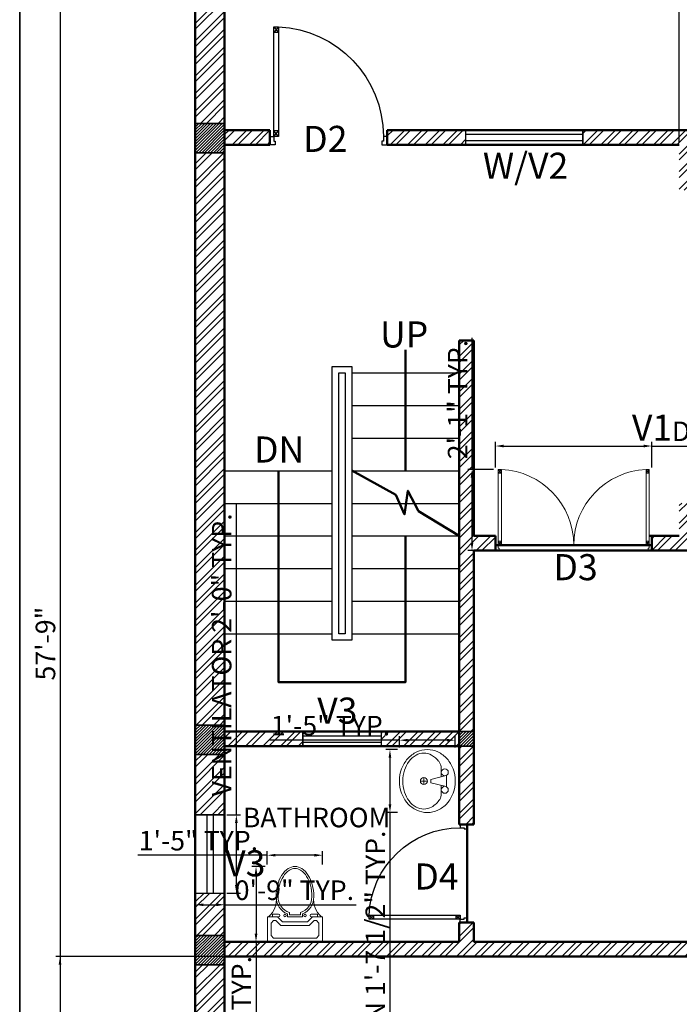
# Model space of a CAD drawing. Units: millimetres. Extents: x 20768 to 23556, y 50760 to 52704.
# Tile 24 of 36: x 21272 to 21474, y 52066 to 52368. Entities that reach past the tile are written whole.
import ezdxf

# ---------------------------------------------------------------- set-up
doc = ezdxf.new("R2010")
doc.units = ezdxf.units.MM
for name, color, linetype, lineweight in [('A-ANNO-TTLB', 7, 'Continuous', 35), ('A-AREA-IDEN', 40, 'Continuous', 18), ('A-DOOR', 3, 'Continuous', 25), ('A-FLOR-STRS', 11, 'Continuous', 25), ('A-FURN', 8, 'Continuous', 18), ('A-GLAZ', 4, 'Continuous', 25), ('A-WALL', 7, 'Continuous', 50), ('A-WALL-PATT', 8, 'Continuous', 13), ('S-ANNO-DIMS', 2, 'Continuous', 18), ('S-COLS', 20, 'Continuous', 35)]:
    doc.layers.add(name, color=color, linetype=linetype, lineweight=lineweight)
doc.styles.get("Standard").update_dxf_attribs({"font": 'arial.ttf'})
doc.dimstyles.new('ISO-25', dxfattribs={"dimtxt": 6, "dimasz": 2.5, "dimexe": 1.25, "dimexo": 0.625, "dimtad": 1, "dimdec": 0, "dimlunit": 3, "dimtxsty": 'Standard', "dimcen": 2.5, "dimadec": 0, "dimazin": 0, "dimtfac": 1, "dimtdec": 0, "dimtmove": 0, "dimatfit": 3, "dimfxl": 1, "dimarcsym": 0})
pattern_1 = [(45, (345.4904, 0), (-0.449012806, 0.449012806), [])]
pattern_2 = [(45, (-37.4434, 0), (-2.69407684, 2.69407684), []), (45, (-35.6473, 0), (-2.69407684, 2.69407684), [])]

# ---------------------------------------------------------------- blocks, each defined once
blk = doc.blocks.new('Puerta 01')
for p, q in [((-0.7745, -0.0264), (-0.7368, -0.0584)), ((-0.7745, -0.0584), (-0.7368, -0.0264)), ((-0.7368, -0.0584), (-0.7368, -0.0264)), ((-0.028, -0.0584), (-0.0657, -0.0264)), ((-0.028, -0.0264), (-0.0657, -0.0584)), ((-0.0657, -0.0584), (-0.0657, -0.0264))]:
    blk.add_line(p, q)
for points in [[(-0.028, 0), (-0.028, -0.0264), (0.004, -0.0264), (0.004, -0.036), (0.028, -0.036), (0.028, 0)], [(-0.028, -0.0264), (-0.7745, -0.0264), (-0.7745, -0.0584), (-0.028, -0.0584)], [(0.004, -0.7736), (0.004, -0.764), (0.028, -0.764), (0.028, -0.8), (-0.028, -0.8), (-0.028, -0.7736)]]:
    blk.add_lwpolyline(points, close=True)
blk.add_arc((-0.028, -0.0264), 0.7472, 182.45453, 270)
blk = doc.blocks.new('md')
for p, q in [((21281.56, 52416.74), (21282.55, 52415.57)), ((21282.55, 52416.74), (21281.56, 52415.57)), ((21327.92, 52416.74), (21326.93, 52415.57)), ((21326.93, 52416.74), (21327.92, 52415.57)), ((21282.55, 52415.57), (21281.56, 52415.57)), ((21326.93, 52415.57), (21327.92, 52415.57)), ((21282.55, 52393.58), (21281.56, 52394.75)), ((21281.56, 52393.58), (21282.55, 52394.75)), ((21282.55, 52394.75), (21281.56, 52394.75)), ((21326.93, 52393.58), (21327.92, 52394.75)), ((21327.92, 52393.58), (21326.93, 52394.75)), ((21326.93, 52394.75), (21327.92, 52394.75))]:
    blk.add_line(p, q)
for points in [[(21281.56, 52393.58), (21281.56, 52416.74), (21282.55, 52416.74), (21282.55, 52393.58)], [(21327.92, 52393.58), (21327.92, 52416.74), (21326.93, 52416.74), (21326.93, 52393.58)], [(21280.74, 52393.58), (21281.56, 52393.58), (21281.56, 52392.59), (21281.86, 52392.59), (21281.86, 52391.84), (21280.74, 52391.84)], [(21328.74, 52393.58), (21327.92, 52393.58), (21327.92, 52392.59), (21327.62, 52392.59), (21327.62, 52391.84), (21328.74, 52391.84)]]:
    blk.add_lwpolyline(points, close=True)
for centre, start, end in [((21281.56, 52393.58), 0, 87.5455), ((21327.92, 52393.58), 92.4545, 180)]:
    blk.add_arc(centre, 23.18, start, end)
blk = doc.blocks.new('A$C0E746A5D')
for p, q in [((0.1052, 0.332), (0.1052, 0.2695)), ((0.0657, 0.276), (0.0657, 0.1972)), ((0.0789, 0.276), (0.184, 0.2497)), ((0.184, 0.2235), (0.0789, 0.1972)), ((0.184, 0.2497), (0.184, 0.2235)), ((0.2103, 0.2366), (0.2629, 0.2366)), ((0.2366, 0.2629), (0.2366, 0.2103)), ((0.1052, 0.2037), (0.1052, 0.141))]:
    blk.add_line(p, q)
for centre in [(0.0789, 0.3023), (0.2366, 0.2366), (0.0789, 0.1709)]:
    blk.add_circle(centre, 0.0263)
for centre, radius, start, end in [((0.2214, 0.2619), 0.2138, 114.98506, 138.36645), ((0.2103, 0.2856), 0.1876, 89.99999, 114.98508), ((0.2366, 0.3272), 0.1197, 90, 118.9112), ((0.2103, 0.2856), 0.1876, 65.01492, 90.00001), ((0.2366, 0.3272), 0.1197, 61.0888, 90), ((0.1992, 0.2619), 0.2138, 41.63355, 65.01494), ((0.2386, 0.2465), 0.2368, 138.36645, 159.7868), ((0.184, 0.332), 0.0789, 147.74019, 180), ((0.2607, 0.2836), 0.1695, 118.9112, 147.74019), ((0.2125, 0.2836), 0.1695, 36.8699, 61.0888), ((0.1746, 0.2552), 0.2169, 17.25794, 36.8699), ((0.182, 0.2465), 0.2368, 20.2132, 41.63355), ((0.2656, 0.2366), 0.2656, 159.78682, 180), ((0.1148, 0.2366), 0.2795, 0, 17.25794), ((0.155, 0.2366), 0.2656, 0, 20.21318), ((0.2656, 0.2366), 0.2656, 180, 200.21318), ((0.1148, 0.2366), 0.2795, 342.74206, 0), ((0.155, 0.2366), 0.2656, 339.78682, 360), ((0.1746, 0.218), 0.2169, 323.1301, 342.74206), ((0.2386, 0.2267), 0.2368, 200.2132, 221.63355), ((0.184, 0.141), 0.0789, 180, 213.90451), ((0.2986, 0.218), 0.2169, 213.90451, 216.8699), ((0.2607, 0.1896), 0.1695, 216.8699, 241.0888), ((0.2125, 0.1896), 0.1695, 298.9112, 323.1301), ((0.182, 0.2267), 0.2368, 318.36645, 339.7868), ((0.2214, 0.2113), 0.2138, 221.63355, 245.01494), ((0.2103, 0.1876), 0.1876, 245.01492, 270.00001), ((0.2366, 0.146), 0.1197, 241.0888, 270), ((0.2103, 0.1876), 0.1876, 269.99999, 294.98508), ((0.2366, 0.146), 0.1197, 270, 298.9112), ((0.1992, 0.2113), 0.2138, 294.98506, 318.36645)]:
    blk.add_arc(centre, radius, start, end)
blk = doc.blocks.new('A$C098B081F')
for p, q in [((558.8, 762), (0, 762)), ((0, 762), (0, 508)), ((63.5, 723.9), (38.1, 698.5)), ((38.1, 698.5), (38.1, 571.5)), ((495.3, 723.9), (63.5, 723.9)), ((520.7, 698.5), (495.3, 723.9)), ((520.7, 698.5), (520.7, 571.5)), ((558.8, 762), (558.8, 508)), ((136.6, 596.9), (85.8, 546.1)), ((422.2, 596.9), (136.6, 596.9)), ((422.2, 596.9), (473, 546.1)), ((0, 508), (12.7, 508)), ((12.7, 508), (101.6, 508)), ((38.1, 571.5), (63.5, 546.1)), ((50.8, 508), (50.8, 482.6)), ((50.8, 508), (101.6, 508)), ((63.5, 546.1), (85.8, 546.1)), ((152.4, 558.8), (101.6, 508)), ((114.3, 508), (101.6, 508)), ((406.4, 558.8), (152.4, 558.8)), ((203.2, 508), (203.2, 479.4)), ((203.2, 508), (355.6, 508)), ((355.6, 508), (355.6, 479.4)), ((406.4, 558.8), (457.2, 508)), ((444.5, 508), (457.2, 508)), ((508, 508), (457.2, 508)), ((495.3, 546.1), (473, 546.1)), ((495.3, 546.1), (520.7, 571.5)), ((508, 508), (546.1, 508)), ((508, 508), (508, 482.6)), ((558.8, 508), (546.1, 508)), ((50.8, 482.6), (114.3, 482.6)), ((223.2, 488), (223.2, 465.8)), ((223.2, 488), (335.6, 488)), ((335.6, 488), (335.6, 465.8)), ((508, 482.6), (444.5, 482.6))]:
    blk.add_line(p, q)
for centre in [(177.8, 495.3), (381, 495.3)]:
    blk.add_circle(centre, 12.7)
for centre, radius, start, end in [((-137.5, 335.8), 228.5, 352.20108, 48.91101), ((114.3, 495.3), 12.7, 270, 90), ((444.5, 495.3), 12.7, 90, 270), ((696.3, 335.8), 228.5, 131.08899, 187.79892), ((279.4, 304.8), 190.5, 113.57818, 180), ((279.4, 304.8), 170.5, 109.24564, 180), ((279.4, 304.8), 170.5, 0, 70.75436), ((279.4, 304.8), 190.5, 0, 66.42182), ((574.9, 304.8), 486, 180.00004, 194.51425), ((574.9, 304.8), 466, 180.00004, 194.51425), ((-16.1, 304.8), 466, 345.48575, 359.99996), ((-16.1, 304.8), 486, 345.48575, 359.99996), ((429.2, 267.1), 335.5, 194.51426, 212.00539), ((429.2, 267.1), 315.5, 194.51426, 212.00539), ((337.2, 209.6), 207, 212.00541, 236.46588), ((221.6, 209.6), 207, 303.53412, 327.99459), ((129.6, 267.1), 315.5, 327.99461, 345.48574), ((129.6, 267.1), 335.5, 327.99461, 345.48574), ((337.2, 209.6), 227, 212.00541, 236.46588), ((279.4, 122.4), 122.4, 236.46593, 269.99995), ((279.4, 122.4), 102.4, 236.46593, 269.99995), ((279.4, 122.4), 102.4, 270.00005, 303.53407), ((279.4, 122.4), 122.4, 270.00005, 303.53407), ((221.6, 209.6), 227, 303.53412, 327.99459)]:
    blk.add_arc(centre, radius, start, end)
blk = doc.blocks.new('WIN-PLAN-A')
blk.add_line((36, 4.5), (36, 0))
blk.add_lwpolyline([(36, 4.5), (0, 4.5), (0, 0), (36, 0)], close=True)
blk = doc.blocks.new('WIN-PLAN-B')
blk.add_line((0, 4.5), (0, 0))
blk.add_lwpolyline([(0, 4.5), (24, 4.5), (24, 0), (0, 0)], close=True)
blk = doc.blocks.new('WIN-PLAN-D')
blk.add_line((0, 24), (9, 24))
blk.add_lwpolyline([(9, 24), (0, 24), (0, 0), (9, 0)], close=True)
blk = doc.blocks.new('*D181')
at = {"layer": 'Defpoints', "color": 0, "transparency": 16777216}
for p in [(21334.74, 52123.9), (21338.34, 52123.9), (21334.74, 52099.9)]:
    blk.add_point(p, dxfattribs=at)
at = {"layer": 'S-ANNO-DIMS', "color": 0, "lineweight": -2, "transparency": 16777216}
for p, q in [((21338.34, 52123.9), (21338.34, 52219.49)), ((21335.37, 52123.9), (21339.59, 52123.9)), ((21338.34, 52102.4), (21338.34, 52121.4)), ((21335.37, 52099.9), (21339.59, 52099.9))]:
    blk.add_line(p, q, dxfattribs=at)
at = {"layer": 'S-ANNO-DIMS', "color": 0, "transparency": 16777216}
for points in [[(21337.92, 52121.4), (21338.76, 52121.4), (21338.34, 52123.9)], [(21337.92, 52102.4), (21338.76, 52102.4), (21338.34, 52099.9)]]:
    blk.add_solid(points, dxfattribs=at)
at = {"layer": 'S-ANNO-DIMS', "color": 0, "transparency": 16777216, "insert": (21334.61, 52172.94), "char_height": 6, "attachment_point": 5, "rotation": 90}
blk.add_mtext('VENTILATOR 2\'-0" TYP.', dxfattribs=at)
blk = doc.blocks.new('*D182')
at = {"layer": 'Defpoints', "color": 0, "transparency": 16777216}
for p in [(21325.74, 52099.9), (21334.74, 52099.9), (21334.74, 52096.3)]:
    blk.add_point(p, dxfattribs=at)
at = {"layer": 'S-ANNO-DIMS', "color": 0, "lineweight": -2, "transparency": 16777216}
for p, q in [((21325.74, 52099.27), (21325.74, 52095.05)), ((21334.74, 52099.27), (21334.74, 52095.05)), ((21328.24, 52096.3), (21332.24, 52096.3)), ((21334.74, 52096.3), (21375.06, 52096.3))]:
    blk.add_line(p, q, dxfattribs=at)
at = {"layer": 'S-ANNO-DIMS', "color": 0, "transparency": 16777216}
for points in [[(21328.24, 52096.71), (21328.24, 52095.88), (21325.74, 52096.3)], [(21332.24, 52096.71), (21332.24, 52095.88), (21334.74, 52096.3)]]:
    blk.add_solid(points, dxfattribs=at)
at = {"layer": 'S-ANNO-DIMS', "color": 0, "transparency": 16777216, "insert": (21356.15, 52099.99), "char_height": 6, "attachment_point": 5}
blk.add_mtext('0\'-9" TYP.', dxfattribs=at)
blk = doc.blocks.new('*D185')
at = {"layer": 'Defpoints', "color": 0, "transparency": 16777216}
for p in [(21465.84, 52236.99), (21417.84, 52229.79), (21465.84, 52229.79)]:
    blk.add_point(p, dxfattribs=at)
at = {"layer": 'S-ANNO-DIMS', "color": 0, "lineweight": -2, "transparency": 16777216}
for p, q in [((21417.84, 52230.42), (21417.84, 52238.24)), ((21465.84, 52230.42), (21465.84, 52238.24)), ((21420.34, 52236.99), (21463.34, 52236.99)), ((21465.84, 52236.99), (21583.18, 52236.99))]:
    blk.add_line(p, q, dxfattribs=at)
at = {"layer": 'S-ANNO-DIMS', "color": 0, "transparency": 16777216}
for points in [[(21420.34, 52237.41), (21420.34, 52236.58), (21417.84, 52236.99)], [(21463.34, 52237.41), (21463.34, 52236.58), (21465.84, 52236.99)]]:
    blk.add_solid(points, dxfattribs=at)
at = {"layer": 'S-ANNO-DIMS', "color": 0, "transparency": 16777216, "insert": (21525.76, 52240.73), "char_height": 6, "attachment_point": 5}
blk.add_mtext('DOUBLE DOOR D3 4\'-0" TYP.', dxfattribs=at)
blk = doc.blocks.new('*D186')
at = {"layer": 'Defpoints', "color": 0, "transparency": 16777216}
for p in [(21410.64, 52229.79), (21417.84, 52229.79), (21417.84, 52204.9)]:
    blk.add_point(p, dxfattribs=at)
at = {"layer": 'S-ANNO-DIMS', "color": 0, "lineweight": -2, "transparency": 16777216}
for p, q in [((21410.64, 52229.79), (21410.64, 52270.22)), ((21417.21, 52229.79), (21409.39, 52229.79)), ((21410.64, 52207.4), (21410.64, 52227.29)), ((21417.21, 52204.9), (21409.39, 52204.9))]:
    blk.add_line(p, q, dxfattribs=at)
at = {"layer": 'S-ANNO-DIMS', "color": 0, "transparency": 16777216}
for points in [[(21410.22, 52227.29), (21411.05, 52227.29), (21410.64, 52229.79)], [(21410.22, 52207.4), (21411.05, 52207.4), (21410.64, 52204.9)]]:
    blk.add_solid(points, dxfattribs=at)
at = {"layer": 'S-ANNO-DIMS', "color": 0, "transparency": 16777216, "insert": (21407, 52251.26), "char_height": 6, "attachment_point": 5, "rotation": 90}
blk.add_mtext('2\'-1" TYP.', dxfattribs=at)
blk = doc.blocks.new('*D197')
at = {"layer": 'Defpoints', "color": 0, "transparency": 16777216}
for p in [(21388.36, 52143.88), (21385.47, 52124.58), (21388.36, 52124.58)]:
    blk.add_point(p, dxfattribs=at)
at = {"layer": 'S-ANNO-DIMS', "color": 0, "lineweight": -2, "transparency": 16777216}
for p, q in [((21387.74, 52143.88), (21384.22, 52143.88)), ((21385.47, 52141.38), (21385.47, 52127.08)), ((21387.74, 52124.58), (21384.22, 52124.58)), ((21385.47, 52124.58), (21385.47, 52015.08))]:
    blk.add_line(p, q, dxfattribs=at)
at = {"layer": 'S-ANNO-DIMS', "color": 0, "transparency": 16777216}
for points in [[(21385.05, 52141.38), (21385.88, 52141.38), (21385.47, 52143.88)], [(21385.05, 52127.08), (21385.88, 52127.08), (21385.47, 52124.58)]]:
    blk.add_solid(points, dxfattribs=at)
at = {"layer": 'S-ANNO-DIMS', "color": 0, "transparency": 16777216, "insert": (21381.74, 52068.58), "char_height": 6, "attachment_point": 5, "rotation": 90}
blk.add_mtext('WASH BASIN 1\'-7 1/2" TYP.', dxfattribs=at)
blk = doc.blocks.new('*D198')
at = {"layer": 'Defpoints', "color": 0, "transparency": 16777216}
for p in [(21388.36, 52146.77), (21388.36, 52143.88), (21405.51, 52143.88)]:
    blk.add_point(p, dxfattribs=at)
at = {"layer": 'S-ANNO-DIMS', "color": 0, "lineweight": -2, "transparency": 16777216}
for p, q in [((21388.36, 52144.5), (21388.36, 52148.02)), ((21405.51, 52144.5), (21405.51, 52148.02)), ((21388.36, 52146.77), (21348.6, 52146.77)), ((21403.01, 52146.77), (21390.86, 52146.77))]:
    blk.add_line(p, q, dxfattribs=at)
at = {"layer": 'S-ANNO-DIMS', "color": 0, "transparency": 16777216}
for points in [[(21390.86, 52147.19), (21390.86, 52146.36), (21388.36, 52146.77)], [(21403.01, 52147.19), (21403.01, 52146.36), (21405.51, 52146.77)]]:
    blk.add_solid(points, dxfattribs=at)
at = {"layer": 'S-ANNO-DIMS', "color": 0, "transparency": 16777216, "insert": (21367.23, 52150.46), "char_height": 6, "attachment_point": 5}
blk.add_mtext('1\'-5" TYP.', dxfattribs=at)
blk = doc.blocks.new('*D199')
at = {"layer": 'Defpoints', "color": 0, "transparency": 16777216}
for p in [(21347.84, 52108.03), (21344.37, 52084.9), (21347.84, 52084.9)]:
    blk.add_point(p, dxfattribs=at)
at = {"layer": 'S-ANNO-DIMS', "color": 0, "lineweight": -2, "transparency": 16777216}
for p, q in [((21347.22, 52108.03), (21343.12, 52108.03)), ((21344.37, 52105.53), (21344.37, 52087.4)), ((21347.22, 52084.9), (21343.12, 52084.9)), ((21344.37, 52084.9), (21344.37, 52023.37))]:
    blk.add_line(p, q, dxfattribs=at)
at = {"layer": 'S-ANNO-DIMS', "color": 0, "transparency": 16777216}
for points in [[(21343.96, 52105.53), (21344.79, 52105.53), (21344.37, 52108.03)], [(21343.96, 52087.4), (21344.79, 52087.4), (21344.37, 52084.9)]]:
    blk.add_solid(points, dxfattribs=at)
at = {"layer": 'S-ANNO-DIMS', "color": 0, "transparency": 16777216, "insert": (21340.65, 52052.89), "char_height": 6, "attachment_point": 5, "rotation": 90}
blk.add_mtext('WC 1\'-11" TYP.', dxfattribs=at)
blk = doc.blocks.new('*D200')
at = {"layer": 'Defpoints', "color": 0, "transparency": 16777216}
for p in [(21347.84, 52111.5), (21347.84, 52108.03), (21364.81, 52108.03)]:
    blk.add_point(p, dxfattribs=at)
at = {"layer": 'S-ANNO-DIMS', "color": 0, "lineweight": -2, "transparency": 16777216}
for p, q in [((21347.84, 52111.5), (21308.08, 52111.5)), ((21347.84, 52108.66), (21347.84, 52112.75)), ((21362.31, 52111.5), (21350.34, 52111.5)), ((21364.81, 52108.66), (21364.81, 52112.75))]:
    blk.add_line(p, q, dxfattribs=at)
at = {"layer": 'S-ANNO-DIMS', "color": 0, "transparency": 16777216}
for points in [[(21350.34, 52111.92), (21350.34, 52111.08), (21347.84, 52111.5)], [(21362.31, 52111.92), (21362.31, 52111.08), (21364.81, 52111.5)]]:
    blk.add_solid(points, dxfattribs=at)
at = {"layer": 'S-ANNO-DIMS', "color": 0, "transparency": 16777216, "insert": (21326.71, 52115.19), "char_height": 6, "attachment_point": 5}
blk.add_mtext('1\'-5" TYP.', dxfattribs=at)
blk = doc.blocks.new('*D211')
at = {"layer": 'Defpoints', "color": 0, "transparency": 16777216}
for p in [(21325.74, 52522.9), (21284.24, 51829.9), (21325.74, 51829.9)]:
    blk.add_point(p, dxfattribs=at)
at = {"layer": 'S-ANNO-DIMS', "color": 0, "lineweight": -2, "transparency": 16777216}
for p, q in [((21325.12, 52522.9), (21282.99, 52522.9)), ((21284.24, 52520.4), (21284.24, 51832.4)), ((21325.12, 51829.9), (21282.99, 51829.9))]:
    blk.add_line(p, q, dxfattribs=at)
at = {"layer": 'S-ANNO-DIMS', "color": 0, "transparency": 16777216}
for points in [[(21283.82, 52520.4), (21284.66, 52520.4), (21284.24, 52522.9)], [(21283.82, 51832.4), (21284.66, 51832.4), (21284.24, 51829.9)]]:
    blk.add_solid(points, dxfattribs=at)
at = {"layer": 'S-ANNO-DIMS', "color": 0, "transparency": 16777216, "insert": (21280.55, 52176.4), "char_height": 6, "attachment_point": 5, "rotation": 90}
blk.add_mtext('57\'-9"', dxfattribs=at)
blk = doc.blocks.new('*D212')
at = {"layer": 'Defpoints', "color": 0, "transparency": 16777216}
for p in [(21334.74, 52080.4), (21284.24, 51900.4), (21334.74, 51900.4)]:
    blk.add_point(p, dxfattribs=at)
at = {"layer": 'S-ANNO-DIMS', "color": 0, "lineweight": -2, "transparency": 16777216}
for p, q in [((21334.12, 52080.4), (21282.99, 52080.4)), ((21284.24, 52077.9), (21284.24, 51902.9)), ((21334.12, 51900.4), (21282.99, 51900.4))]:
    blk.add_line(p, q, dxfattribs=at)
at = {"layer": 'S-ANNO-DIMS', "color": 0, "transparency": 16777216}
for points in [[(21283.82, 52077.9), (21284.66, 52077.9), (21284.24, 52080.4)], [(21283.82, 51902.9), (21284.66, 51902.9), (21284.24, 51900.4)]]:
    blk.add_solid(points, dxfattribs=at)
at = {"layer": 'S-ANNO-DIMS', "color": 0, "transparency": 16777216, "insert": (21280.55, 51990.4), "char_height": 6, "attachment_point": 5, "rotation": 90}
blk.add_mtext('15\'-0"', dxfattribs=at)
blk = doc.blocks.new('*D215')
at = {"layer": 'Defpoints', "color": 0, "transparency": 16777216}
for p in [(21474.24, 52564.4), (21334.74, 52329.4), (21474.24, 52329.4)]:
    blk.add_point(p, dxfattribs=at)
at = {"layer": 'S-ANNO-DIMS', "color": 0, "lineweight": -2, "transparency": 16777216}
for p, q in [((21334.74, 52330.02), (21334.74, 52565.65)), ((21337.24, 52564.4), (21471.74, 52564.4)), ((21474.24, 52330.02), (21474.24, 52565.65))]:
    blk.add_line(p, q, dxfattribs=at)
at = {"layer": 'S-ANNO-DIMS', "color": 0, "transparency": 16777216}
for points in [[(21337.24, 52564.81), (21337.24, 52563.98), (21334.74, 52564.4)], [(21471.74, 52564.81), (21471.74, 52563.98), (21474.24, 52564.4)]]:
    blk.add_solid(points, dxfattribs=at)
at = {"layer": 'S-ANNO-DIMS', "color": 0, "transparency": 16777216, "insert": (21404.49, 52568.12), "char_height": 6, "attachment_point": 5}
blk.add_mtext('11\'-7 1/2"', dxfattribs=at)

msp = doc.modelspace()

# ---------------------------------------------------------------- hatches: boundary and pattern name
at = {"layer": 'A-WALL-PATT'}
h = msp.add_hatch(dxfattribs=at)
h.set_pattern_fill('ANSI32', color=256, scale=0.4)
h.set_pattern_definition(pattern_2)
h.paths.add_polyline_path([(21334.74, 52513.9), (21325.74, 52513.9), (21325.74, 52335.9), (21334.74, 52335.9)])
h = msp.add_hatch(dxfattribs=at)
h.set_pattern_fill('ANSI31', color=256, scale=0.2)
h.set_pattern_definition(pattern_1)
h.paths.add_polyline_path([(21334.74, 52335.9), (21325.74, 52335.9), (21325.74, 52326.9), (21334.74, 52326.9)])
h = msp.add_hatch(dxfattribs=at)
h.set_pattern_fill('ANSI32', color=256, scale=0.4)
h.set_pattern_definition(pattern_2)
h.paths.add_polyline_path([(21348.64, 52333.9), (21334.74, 52333.9), (21334.74, 52329.4), (21348.64, 52329.4), (21348.64, 52331.92)])
h = msp.add_hatch(dxfattribs=at)
h.set_pattern_fill('ANSI32', color=256, scale=0.4)
h.set_pattern_definition(pattern_2)
h.paths.add_polyline_path([(21408.64, 52333.9), (21384.64, 52333.9), (21384.64, 52329.4), (21408.64, 52329.4)])
h = msp.add_hatch(dxfattribs=at)
h.set_pattern_fill('ANSI32', color=256, scale=0.4)
h.set_pattern_definition(pattern_2)
h.paths.add_polyline_path([(21550.74, 52333.9), (21444.64, 52333.9), (21444.64, 52329.4), (21474.24, 52329.4), (21474.24, 52315.5), (21476.76, 52315.5), (21478.74, 52315.5), (21478.74, 52329.4), (21550.74, 52329.4)])
h = msp.add_hatch(dxfattribs=at)
h.set_pattern_fill('ANSI32', color=256, scale=0.4)
h.set_pattern_definition(pattern_2)
h.paths.add_polyline_path([(21334.74, 52326.9), (21325.74, 52326.9), (21325.74, 52151.4), (21334.74, 52151.4)])
h = msp.add_hatch(dxfattribs=at)
h.set_pattern_fill('ANSI32', color=256, scale=0.4)
h.set_pattern_definition(pattern_2)
h.paths.add_polyline_path([(21411.24, 52204.9), (21417.84, 52204.9), (21417.84, 52209.4), (21411.24, 52209.4), (21411.24, 52269.4), (21406.74, 52269.4), (21406.74, 52149.4), (21411.24, 52149.4)])
h = msp.add_hatch(dxfattribs=at)
h.set_pattern_fill('ANSI32', color=256, scale=0.4)
h.set_pattern_definition(pattern_2)
h.paths.add_polyline_path([(21486.24, 52209.4), (21478.74, 52209.4), (21478.74, 52219.5), (21474.24, 52219.5), (21474.24, 52209.4), (21465.84, 52209.4), (21465.84, 52204.9), (21486.24, 52204.9)])
h = msp.add_hatch(dxfattribs=at)
h.set_pattern_fill('ANSI31', color=256, scale=0.2)
h.set_pattern_definition(pattern_1)
h.paths.add_polyline_path([(21334.74, 52151.4), (21325.74, 52151.4), (21325.74, 52142.4), (21334.74, 52142.4)])
h = msp.add_hatch(dxfattribs=at)
h.set_pattern_fill('ANSI32', color=256, scale=0.4)
h.set_pattern_definition(pattern_2)
h.paths.add_polyline_path([(21358.74, 52149.4), (21334.74, 52149.4), (21334.74, 52144.9), (21358.74, 52144.9)])
h = msp.add_hatch(dxfattribs=at)
h.set_pattern_fill('ANSI32', color=256, scale=0.4)
h.set_pattern_definition(pattern_2)
h.paths.add_polyline_path([(21406.74, 52149.4), (21382.74, 52149.4), (21382.74, 52144.9), (21406.74, 52144.9)])
h = msp.add_hatch(dxfattribs=at)
h.set_pattern_fill('ANSI31', color=256, scale=0.2)
h.set_pattern_definition(pattern_1)
h.paths.add_polyline_path([(21411.24, 52149.4), (21406.74, 52149.4), (21406.74, 52144.9), (21411.24, 52144.9)])
h = msp.add_hatch(dxfattribs=at)
h.set_pattern_fill('ANSI32', color=256, scale=0.4)
h.set_pattern_definition(pattern_2)
h.paths.add_polyline_path([(21411.24, 52144.9), (21406.74, 52144.9), (21406.74, 52120.9), (21411.24, 52120.9)])
h = msp.add_hatch(dxfattribs=at)
h.set_pattern_fill('ANSI32', color=256, scale=0.4)
h.set_pattern_definition(pattern_2)
h.paths.add_polyline_path([(21334.74, 52142.4), (21325.74, 52142.4), (21325.74, 52123.9), (21334.74, 52123.9)])
h = msp.add_hatch(dxfattribs=at)
h.set_pattern_fill('ANSI32', color=256, scale=0.4)
h.set_pattern_definition(pattern_2)
h.paths.add_polyline_path([(21334.74, 52099.9), (21325.74, 52099.9), (21325.74, 52086.9), (21334.74, 52086.9)])
h = msp.add_hatch(dxfattribs=at)
h.set_pattern_fill('ANSI32', color=256, scale=0.4)
h.set_pattern_definition(pattern_2)
h.paths.add_polyline_path([(21508.74, 52084.9), (21411.24, 52084.9), (21411.24, 52090.9), (21406.74, 52090.9), (21406.74, 52084.9), (21334.74, 52084.9), (21334.74, 52080.4), (21508.74, 52080.4)])
h = msp.add_hatch(dxfattribs=at)
h.set_pattern_fill('ANSI31', color=256, scale=0.2)
h.set_pattern_definition(pattern_1)
h.paths.add_polyline_path([(21334.74, 52086.9), (21325.74, 52086.9), (21325.74, 52077.9), (21334.74, 52077.9)])
h = msp.add_hatch(dxfattribs=at)
h.set_pattern_fill('ANSI32', color=256, scale=0.4)
h.set_pattern_definition(pattern_2)
h.paths.add_polyline_path([(21334.74, 52077.9), (21325.74, 52077.9), (21325.74, 51902.4), (21334.74, 51902.4)])

# ---------------------------------------------------------------- linework, layer by layer
at = {"layer": 'A-ANNO-TTLB'}
msp.add_line((21271.86, 52703.98), (21271.86, 51623.53), dxfattribs=at)
at = {"layer": 'A-FLOR-STRS'}
for p, q in [((21373.74, 52259.4), (21406.74, 52259.4)), ((21373.74, 52249.4), (21406.74, 52249.4)), ((21373.74, 52239.4), (21406.74, 52239.4)), ((21334.74, 52229.4), (21367.74, 52229.4)), ((21373.74, 52229.4), (21406.74, 52229.4)), ((21334.74, 52219.4), (21367.74, 52219.4)), ((21373.74, 52219.4), (21406.74, 52219.4)), ((21334.74, 52209.4), (21367.74, 52209.4)), ((21373.74, 52209.4), (21406.74, 52209.4)), ((21334.74, 52199.4), (21367.74, 52199.4)), ((21373.74, 52199.4), (21406.74, 52199.4)), ((21334.74, 52189.4), (21367.74, 52189.4)), ((21373.74, 52189.4), (21406.74, 52189.4)), ((21334.74, 52179.4), (21367.74, 52179.4)), ((21373.74, 52179.4), (21406.74, 52179.4))]:
    msp.add_line(p, q, dxfattribs=at)
for points in [[(21373.74, 52177.4), (21367.74, 52177.4), (21367.74, 52261.4), (21373.74, 52261.4)], [(21371.74, 52179.4), (21369.74, 52179.4), (21369.74, 52259.4), (21371.74, 52259.4)]]:
    msp.add_lwpolyline(points, close=True, dxfattribs=at)
at = {"layer": 'A-GLAZ'}
for p, q in [((21408.64, 52333.9), (21408.64, 52329.4)), ((21408.64, 52332.65), (21444.64, 52332.65)), ((21408.64, 52330.65), (21444.64, 52330.65)), ((21358.74, 52148.15), (21382.74, 52148.15)), ((21382.74, 52149.4), (21382.74, 52144.9)), ((21358.74, 52146.15), (21382.74, 52146.15)), ((21329.24, 52123.9), (21329.24, 52099.9)), ((21331.24, 52123.9), (21331.24, 52099.9)), ((21325.74, 52099.9), (21334.74, 52099.9))]:
    msp.add_line(p, q, dxfattribs=at)
at = {"layer": 'A-WALL'}
for p, q in [((21325.74, 52522.9), (21325.74, 51829.9)), ((21334.74, 52513.9), (21334.74, 51829.9)), ((21334.74, 52333.9), (21348.64, 52333.9)), ((21348.64, 52333.9), (21348.64, 52329.4)), ((21384.64, 52333.9), (21384.64, 52329.4)), ((21384.64, 52333.9), (21550.74, 52333.9)), ((21334.74, 52329.4), (21348.64, 52329.4)), ((21384.64, 52329.4), (21474.24, 52329.4)), ((21406.74, 52269.4), (21406.74, 52120.9)), ((21406.74, 52269.4), (21411.24, 52269.4)), ((21411.24, 52269.4), (21411.24, 52209.4)), ((21390.24, 52266.45), (21390.24, 52229.4)), ((21411.24, 52209.4), (21417.84, 52209.4)), ((21417.84, 52209.4), (21417.84, 52204.9)), ((21465.24, 52209.4), (21474.24, 52209.4)), ((21465.84, 52209.4), (21465.84, 52204.9)), ((21411.24, 52204.9), (21411.24, 52120.9)), ((21411.24, 52204.9), (21418.95, 52204.9)), ((21417.84, 52206.63), (21465.84, 52206.63)), ((21417.84, 52204.9), (21465.84, 52204.9)), ((21465.84, 52204.9), (21550.74, 52204.9)), ((21334.74, 52149.4), (21406.74, 52149.4)), ((21334.74, 52144.9), (21406.74, 52144.9)), ((21406.74, 52120.9), (21411.24, 52120.9)), ((21409.14, 52120.9), (21409.14, 52090.9)), ((21406.74, 52090.9), (21406.74, 52084.9)), ((21406.74, 52090.9), (21411.24, 52090.9)), ((21411.24, 52090.9), (21411.24, 52084.9)), ((21334.74, 52084.9), (21406.74, 52084.9)), ((21411.24, 52084.9), (21508.74, 52084.9)), ((21334.74, 52080.4), (21508.74, 52080.4))]:
    msp.add_line(p, q, dxfattribs=at)
for points in [[(21390.24, 52209.4), (21390.24, 52164.58), (21351.24, 52164.58), (21351.24, 52229.4)], [(21406.74, 52209.4), (21394.24, 52216.97), (21390.97, 52223.27), (21389.96, 52216.02), (21387.25, 52222.01), (21373.74, 52229.46)]]:
    msp.add_lwpolyline(points, dxfattribs=at)
at = {"layer": 'S-COLS'}
for points in [[(21334.74, 52335.9), (21325.74, 52335.9), (21325.74, 52326.9), (21334.74, 52326.9)], [(21334.74, 52151.4), (21325.74, 52151.4), (21325.74, 52142.4), (21334.74, 52142.4)], [(21406.74, 52144.9), (21411.24, 52144.9), (21411.24, 52149.4), (21406.74, 52149.4)], [(21334.74, 52086.9), (21325.74, 52086.9), (21325.74, 52077.9), (21334.74, 52077.9)]]:
    msp.add_lwpolyline(points, close=True, dxfattribs=at)

# ---------------------------------------------------------------- block references
at = {"layer": 'A-DOOR', "xscale": -45.00000000000063, "yscale": 45.00000000000063, "zscale": 45.00000000000063, "rotation": 90}
msp.add_blockref('Puerta 01', (21348.64, 52330.66), dxfattribs=at)
at = {"layer": 'A-DOOR', "extrusion": (0, 0, -1), "xscale": 37.50000000000053, "yscale": 37.50000000000053, "zscale": -37.50000000000053, "rotation": 180}
msp.add_blockref('Puerta 01', (-21408.09, 52090.9), dxfattribs=at)
at = {"layer": 'A-FURN'}
msp.add_blockref('md', (137.1, -186.95), dxfattribs=at)
at = {"layer": 'A-FURN', "rotation": 180}
for name, p, xscale, yscale, zscale in [('A$C0E746A5D', (21405.51, 52143.88), 40.7754425969756, 40.7754425969756, 40.7754425969756), ('A$C098B081F', (21364.81, 52108.03), 0.0303586382606966, 0.0303586382606966, 0.0303586382606966)]:
    msp.add_blockref(name, p, dxfattribs=dict(at, xscale=xscale, yscale=yscale, zscale=zscale))
at = {"layer": 'A-GLAZ'}
for name, p in [('WIN-PLAN-A', (21408.64, 52329.4)), ('WIN-PLAN-B', (21358.74, 52144.9)), ('WIN-PLAN-D', (21325.74, 52099.9))]:
    msp.add_blockref(name, p, dxfattribs=at)

# ---------------------------------------------------------------- texts
at = {"layer": 'A-AREA-IDEN', "attachment_point": 1}
for s, width, insert, char_height in [(' D2', 27.5349, (21356.41, 52335.18), 8), ('W/V2', 27.5349, (21413.98, 52326.94), 8), (' UP', 27.5349, (21379.98, 52275.21), 8), (' V1', 27.5349, (21457.26, 52246.62), 8), (' DN', 27.5349, (21341.33, 52239.92), 8), (' D3', 27.5349, (21433.19, 52203.84), 8), (' V3', 27.5349, (21360.72, 52159.84), 8), ('BATHROOM', 49.9521, (21340.33, 52126.06), 6), (' V3', 27.5349, (21332.47, 52113.01), 8), (' D4', 27.5349, (21390.51, 52108.97), 8)]:
    msp.add_mtext_dynamic_manual_height_columns(s, width=width, gutter_width=12.5, heights=[0], dxfattribs=dict(at, insert=insert, char_height=char_height))

# ---------------------------------------------------------------- dimensions: what is measured, and where the dimension line sits
at = {"layer": 'S-ANNO-DIMS'}
dim = msp.add_linear_dim(base=(21474.24, 52564.4), p1=(21334.74, 52329.4), p2=(21474.24, 52329.4), dimstyle='ISO-25', override={"dimdec": 1, "dimlfac": 1, "dimrnd": 0, "dimzin": 1, "dimdsep": 46, "dimlunit": 4, "dimfrac": 2}, dxfattribs=at)
dim.commit()
dim.dimension.update_dxf_attribs({"geometry": '*D215', "text_midpoint": (21404.49, 52568.12)})
for base, p1, p2, picture, middle in [((21284.24, 51829.9), (21325.74, 52522.9), (21325.74, 51829.9), '*D211', (21280.55, 52176.4)), ((21284.24, 51900.4), (21334.74, 52080.4), (21334.74, 51900.4), '*D212', (21280.55, 51990.4))]:
    dim = msp.add_linear_dim(base=base, p1=p1, p2=p2, angle=90, dimstyle='ISO-25', override={"dimdec": 1, "dimlfac": 1, "dimrnd": 0, "dimzin": 1, "dimdsep": 46, "dimlunit": 4, "dimfrac": 2}, dxfattribs=at)
    dim.commit()
    dim.dimension.update_dxf_attribs({"geometry": picture, "text_midpoint": middle})
for base, p1, p2, angle, text, picture, middle in [((21410.64, 52229.79), (21417.84, 52204.9), (21417.84, 52229.79), 90, '<> TYP.', '*D186', (21407, 52251.26)), ((21338.34, 52123.9), (21334.74, 52099.9), (21334.74, 52123.9), 90, 'VENTILATOR <> TYP.', '*D181', (21334.61, 52172.94)), ((21388.3619, 52146.7735), (21405.513, 52143.8792), (21388.3619, 52143.8792), 180, '<> TYP.', '*D198', (21367.2328, 52150.4619)), ((21385.47, 52124.58), (21388.36, 52143.88), (21388.36, 52124.58), 270, 'WASH BASIN <> TYP.', '*D197', (21381.74, 52068.58)), ((21347.84, 52111.5), (21364.81, 52108.03), (21347.84, 52108.03), 180, '<> TYP.', '*D200', (21326.71, 52115.19)), ((21344.37, 52084.9), (21347.84, 52108.03), (21347.84, 52084.9), 270, 'WC <> TYP.', '*D199', (21340.65, 52052.89))]:
    dim = msp.add_linear_dim(base=base, p1=p1, p2=p2, angle=angle, text=text, dimstyle='ISO-25', override={"dimdec": 1, "dimrnd": 0, "dimzin": 1, "dimlunit": 4, "dimfrac": 2}, dxfattribs=at)
    dim.commit()
    dim.dimension.update_dxf_attribs({"geometry": picture, "text_midpoint": middle})
for base, p1, p2, text, picture, middle in [((21465.84, 52236.99), (21417.84, 52229.79), (21465.84, 52229.79), 'DOUBLE DOOR D3 <> TYP.', '*D185', (21525.76, 52240.73)), ((21334.74, 52096.3), (21325.74, 52099.9), (21334.74, 52099.9), '<> TYP.', '*D182', (21356.15, 52099.99))]:
    dim = msp.add_linear_dim(base=base, p1=p1, p2=p2, text=text, dimstyle='ISO-25', override={"dimdec": 1, "dimrnd": 0, "dimzin": 1, "dimlunit": 4, "dimfrac": 2}, dxfattribs=at)
    dim.commit()
    dim.dimension.update_dxf_attribs({"geometry": picture, "text_midpoint": middle})

doc.saveas('drawing.dxf')
